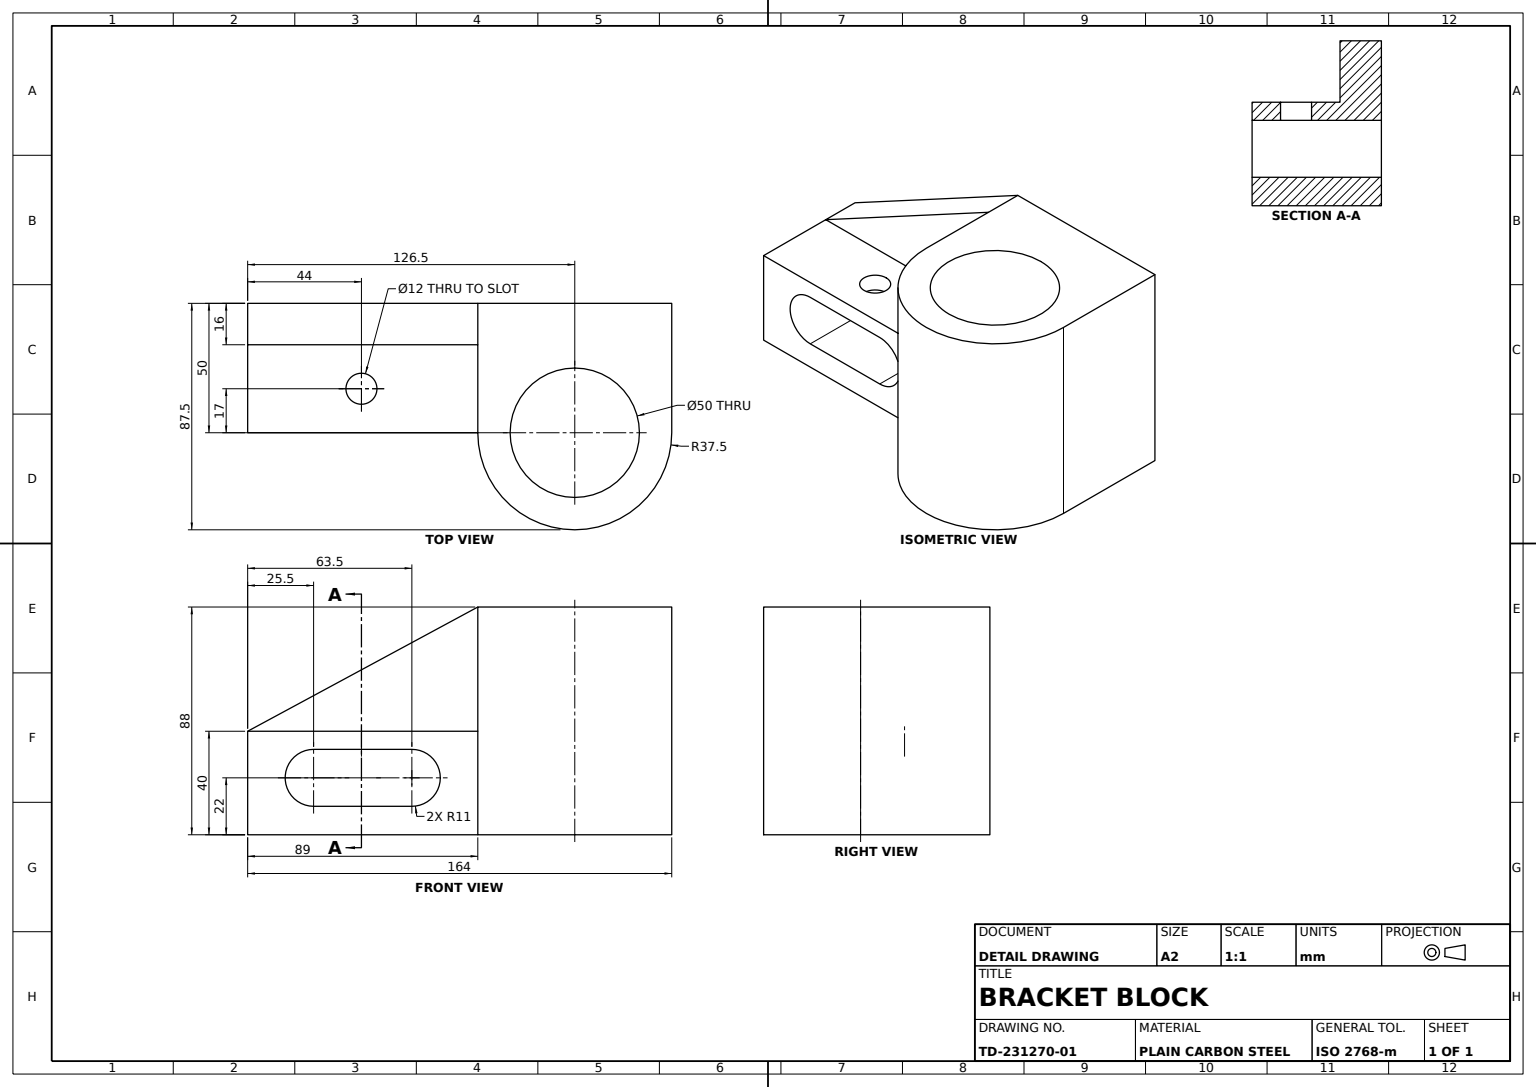
from build123d import *

# Parameters (mm, degrees)
BASE_BLOCK_SKETCH_W       = 89
BASE_BLOCK_SKETCH_H       = 40
BASE_BLOCK_50MM_DEPTH     = 50
ROUNDED_BOSS_44MM_DEPTH   = 44
BOSS_START                = 44
BOSS_EXTENSION_44MM_DEPTH = 44
GUSSET_A_16MM_DEPTH       = 16
RECESS_START              = -4
RECESS_4MM_DEPTH          = 4
PAD_START                 = 4
PAD_4MM_DEPTH             = 4
GUSSET_B_16MM_DEPTH       = 16
BORE_SKETCH_50_R          = 25
BORE_50_DEPTH             = 88
SIDE_SLOT_DEPTH           = 50
HOLE_SKETCH_12_R          = 6
HOLE_12_DEPTH             = 10


with BuildPart() as part:
    # Base Block Sketch → Base Block 50mm (new body)
    with BuildSketch(Plane.XY):
        with Locations((44.5, -20)):
            Rectangle(BASE_BLOCK_SKETCH_W, BASE_BLOCK_SKETCH_H)
    extrude(amount=BASE_BLOCK_50MM_DEPTH)

    # Rounded Boss Sketch → Rounded Boss 44mm (add)
    with BuildSketch(Plane(origin=(0, 0, 0), x_dir=(1, 0, 0), z_dir=(0, 1, 0))):
        with BuildLine():
            Line((89, 0), (89, -16))
            Line((89, -16), (89, -50))
            ThreePointArc((89, -50), (126.5, -87.5), (164, -50))
            Line((164, -50), (164, -16))
            Line((164, -16), (164, 0))
            Line((164, 0), (89, 0))
        make_face()
    extrude(amount=-ROUNDED_BOSS_44MM_DEPTH)

    # Boss Extension Sketch → Boss Extension 44mm (add)
    with BuildSketch(Plane(origin=(0, 0, 0), x_dir=(1, 0, 0), z_dir=(0, 1, 0)).offset(BOSS_START)):
        with BuildLine():
            Line((164, 0), (164, -50))
            ThreePointArc((164, -50), (126.5, -87.5), (89, -50))
            Line((89, -50), (89, 0))
            Line((89, 0), (164, 0))
        make_face()
    extrude(amount=-BOSS_EXTENSION_44MM_DEPTH)

    # Gusset A Sketch → Gusset A 16mm (add)
    with BuildSketch(Plane(origin=(0, 0, 0), x_dir=(-1, 0, 0), z_dir=(0, 0, -1))):
        Polygon((-89, 44), (-89, 0), (0, 0), align=None)
    extrude(amount=-GUSSET_A_16MM_DEPTH)

    # Recess Sketch → Recess 4mm (cut)
    with BuildSketch(Plane.XZ.offset(44).offset(RECESS_START)):
        with BuildLine():
            Line((89, 0), (89, 50))
            ThreePointArc((89, 50), (126.5, 87.5), (164, 50))
            Line((164, 50), (164, 0))
            Line((164, 0), (89, 0))
        make_face()
    extrude(amount=RECESS_4MM_DEPTH, mode=Mode.SUBTRACT)

    # Pad Sketch → Pad 4mm (add)
    with BuildSketch(Plane(origin=(0, 44, 0), x_dir=(1, 0, 0), z_dir=(0, 1, 0)).offset(PAD_START)):
        with BuildLine():
            Line((89, 0), (164, 0))
            Line((164, 0), (164, -50))
            ThreePointArc((164, -50), (126.5, -87.5), (89, -50))
            Line((89, -50), (89, 0))
        make_face()
    extrude(amount=-PAD_4MM_DEPTH)

    # Gusset B Sketch → Gusset B 16mm (add)
    with BuildSketch(Plane(origin=(0, 0, 0), x_dir=(-1, 0, 0), z_dir=(0, 0, -1))):
        Polygon((-89, 48), (-89, 44), (0, 0), align=None)
    extrude(amount=-GUSSET_B_16MM_DEPTH)

    # Bore Sketch Ø50 → Bore Ø50 (cut)
    with BuildSketch(Plane(origin=(0, 48, 0), x_dir=(1, 0, 0), z_dir=(0, 1, 0))):
        with Locations(Location((126.5, -50, 0), (0, 0, 270))):
            Circle(BORE_SKETCH_50_R)
    extrude(amount=-BORE_50_DEPTH, mode=Mode.SUBTRACT)

    # Side Slot Sketch → Side Slot (cut)
    with BuildSketch(Plane.XY.offset(50)):
        with BuildLine():
            Line((25.5, -29), (63.5, -29))
            ThreePointArc((63.5, -29), (74.5, -18), (63.5, -7))
            Line((63.5, -7), (25.5, -7))
            ThreePointArc((25.5, -7), (14.5, -18), (25.5, -29))
        make_face()
    extrude(amount=-SIDE_SLOT_DEPTH, mode=Mode.SUBTRACT)

    # Hole Sketch Ø12 → Hole Ø12 (cut)
    with BuildSketch(Plane(origin=(0, 0, 0), x_dir=(1, 0, 0), z_dir=(0, 1, 0))):
        with Locations(Location((44, -33, 0), (0, 0, 270))):
            Circle(HOLE_SKETCH_12_R)
    extrude(amount=-HOLE_12_DEPTH, mode=Mode.SUBTRACT)


solid = part.part
